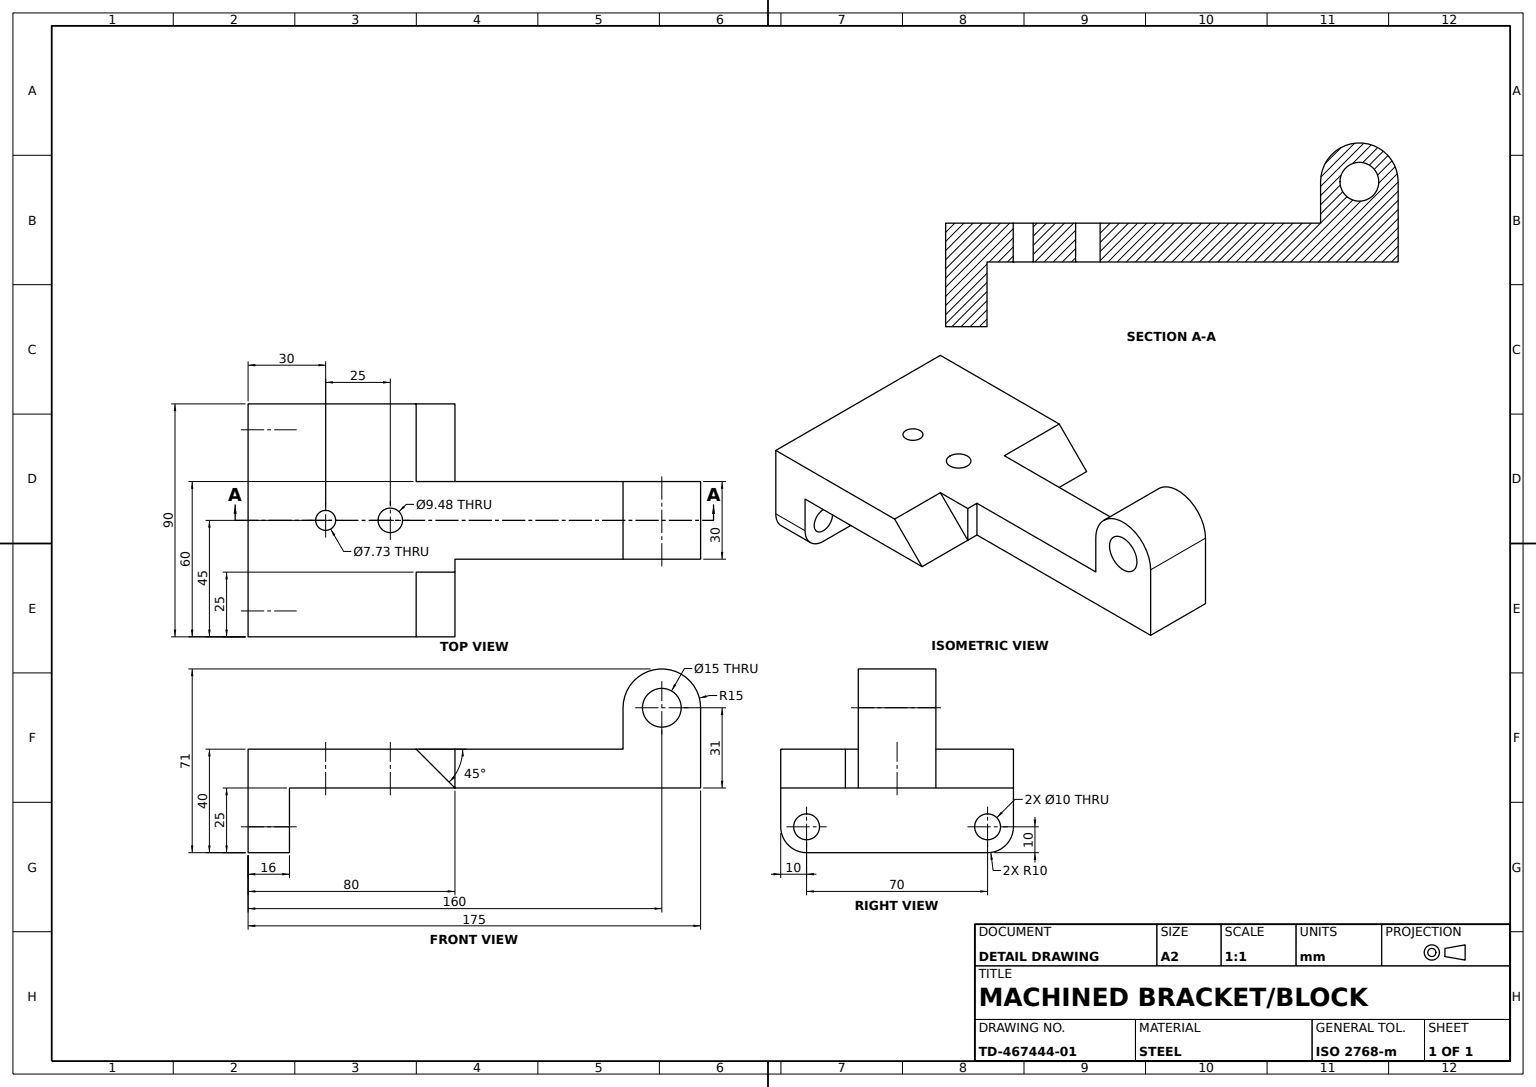
SolidWorks part; units mm, degrees
material "Plain Carbon Steel"
ref_plane "Front Plane" through (0, 0, 0) normal (0, 0, 1) x (1, 0, 0)
ref_plane "Top Plane" through (0, 0, 0) normal (0, 1, 0) x (1, 0, 0)
ref_plane "Right Plane" through (0, 0, 0) normal (1, 0, 0) x (0, 0, -1)
sketch "Base Block Profile" plane through (0, 0, 0) normal (0, 0, 1) x (1, 0, 0)
  line L0 (0, 0) -> (0, -40)
  line L1 (0, -40) -> (16, -40)
  line L2 (16, -40) -> (16, -15)
  line L3 (16, -15) -> (80, -15)
  line L5 (65, 0) -> (0, 0)
  line L6 (80, -15) -> (65, 0)
  dimension "D1" = 80
  dimension "D2" = 45
  dimension "D3" = 40
  dimension "D4" = 16
  dimension "D5" = 15
extrude "Base Block" add sketch "Base Block Profile" along normal mid plane 90
sketch "Step Boss Profile" plane through (0, 0, 0) normal (0, 1, 0) x (1, 0, 0)
  line L1 (65, 45) -> (0, 45) construction
  line L2 (65, -45) -> (65, 45) construction
  line L3 (65, 15) -> (80, 15)
  line L4 (65, 15) -> (65, -20)
  line L5 (65, -20) -> (80, -20)
  line L6 (80, 15) -> (80, -20)
  line L7 (80, -45) -> (80, 45) construction
  dimension "D1" = 35
  dimension "D2" = 30
extrude "Step Boss" add sketch "Step Boss Profile" against normal blind 15
sketch "Arm Profile" plane through (80, 0, 0) normal (1, 0, 0) x (0, 0, -1)
  line L0 (-20, -15) -> (-20, 0) construction
  line L1 (-20, 0) -> (15, 0) construction
  line L2 (15, -15) -> (-15, -15)
  line L3 (15, -15) -> (15, 0)
  line L4 (15, 0) -> (-15, 0)
  line L5 (-15, -15) -> (-15, 0)
  dimension "D1" = 5
extrude "Extension Arm" add sketch "Arm Profile" along normal blind 95
sketch "Hinge Lug Profile" plane through (0, 0, 15) normal (0, 0, 1) x (1, 0, 0)
  line L0 (145, 16) -> (145, -10.792)
  line L1 (175, 16) -> (175, -10.792)
  line L3 (175, 0) -> (175, -15) construction
  line L4 (175, -10.792) -> (145, -10.792)
  line L5 (175, -15) -> (80, -15) construction
  circle A0 centre (160, 16) radius 7.5
  arc A1 (175, 16) -> (145, 16) centre (160, 16) ccw
  dimension "D1" = 30
  dimension "D2" = 15
  dimension "D3" = 4.208
  dimension "D4" = 31
extrude "Hinge Lug" add sketch "Hinge Lug Profile" against normal blind 30
fillet "Edge Fillet R10" radius 10 2 edges at (8, -40, -45) (8, -40, 45)
sketch "Pin Holes Profile" plane through (0, 0, 0) normal (-1, 0, 0) x (0, 0, 1)
  circle A0 centre (-35, -30) radius 5
  circle A1 centre (35, -30) radius 5
  dimension "D1" = 10
  dimension "D2" = 10
extrude "Pin Holes Through" cut sketch "Pin Holes Profile" against normal mid plane 120
sketch "Top Holes Profile" plane through (0, 0, 0) normal (0, 1, 0) x (1, 0, 0)
  line L0 (0, -45) -> (0, 45) construction
  line L2 (145, -15) -> (80, -15) construction
  circle A0 centre (30, 0) radius 3.8627
  circle A1 centre (55, 0) radius 4.7403
  dimension "D3" = 9.4806
  dimension "D4" = 7.7254
  dimension "D1" = 25
  dimension "D2" = 30
  dimension "D5" = 15
extrude "Top Holes Through" cut sketch "Top Holes Profile" against normal mid plane 120
